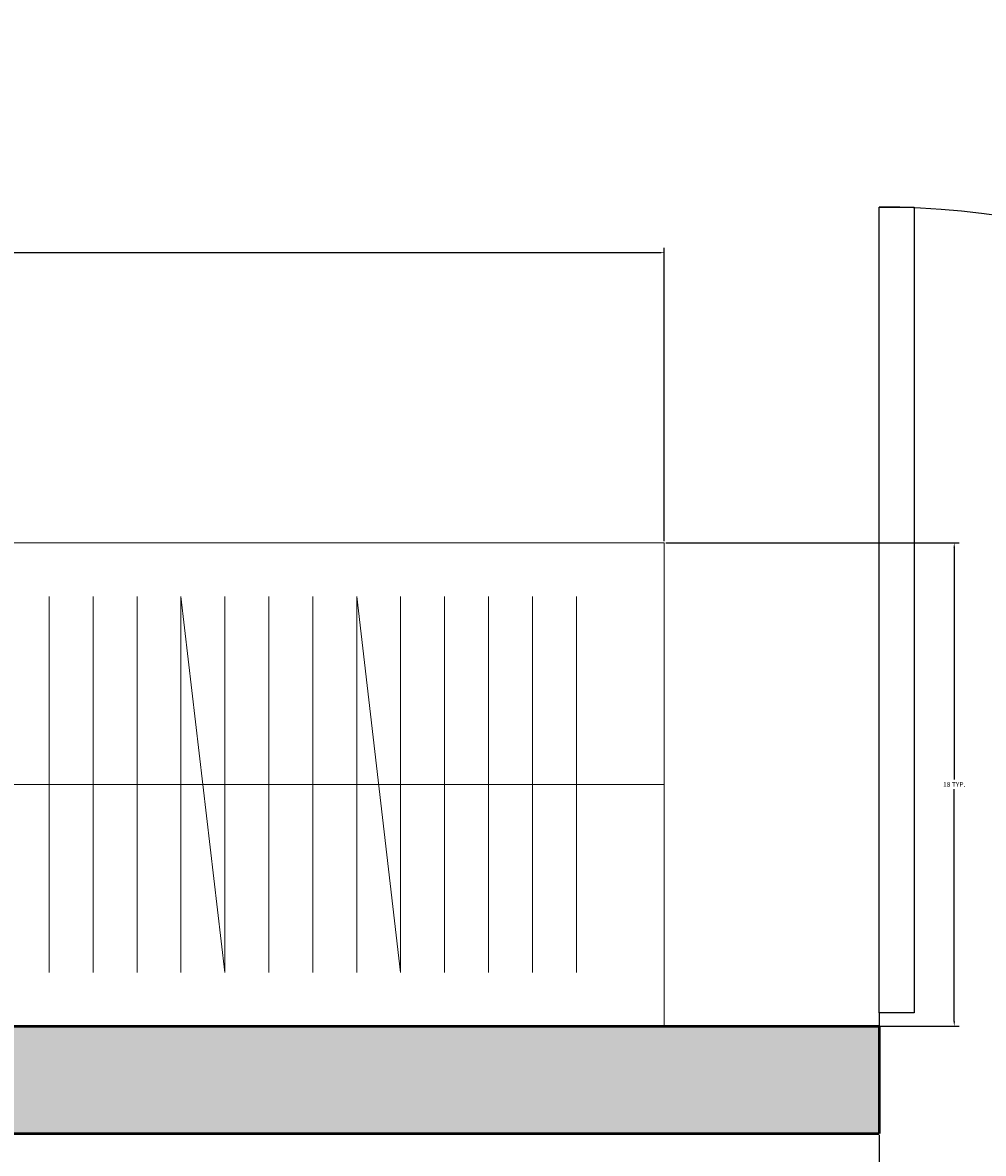
# Model space of a CAD drawing. Units: inches. Extents: x 2307 to 2544, y 2171 to 2540.
# Tile 20 of 52: x 2384 to 2420, y 2387 to 2429. Entities that reach past the tile are written whole.
import ezdxf

# ---------------------------------------------------------------- set-up
doc = ezdxf.new("R2010")
doc.units = ezdxf.units.IN
for name, color, linetype, lineweight in [('A-ANNO-DIMS', 2, 'Continuous', 18), ('A-DOOR', 3, 'Continuous', 25), ('A-FLOR-CASE', 9, 'Continuous', 18), ('A-WALL', 7, 'Continuous', 50)]:
    doc.layers.add(name, color=color, linetype=linetype, lineweight=lineweight)
doc.layers.add('A-WALL-PATT', color=18, linetype='Continuous', lineweight=13, true_color=0x000000)
doc.styles.get("Standard").update_dxf_attribs({"font": 'arial.ttf'})
doc.dimstyles.get("Standard").update_dxf_attribs({"dimtxt": 0.18, "dimasz": 0.18, "dimexe": 0.18, "dimexo": 0.0625, "dimgap": 0.09, "dimtad": 0, "dimtih": 1, "dimtoh": 1, "dimdec": 4, "dimzin": 0, "dimdsep": 46, "dimtxsty": 'Standard', "dimcen": 0.09, "dimadec": 0, "dimazin": 0, "dimtfac": 1, "dimtdec": 4, "dimtofl": 0, "dimtmove": 0, "dimatfit": 3, "dimfxl": 1, "dimtolj": 1, "dimtzin": 0, "dimarcsym": 0})

# ---------------------------------------------------------------- blocks, each defined once
blk = doc.blocks.new('*U13')
for p, q in [((0, 0), (0, -6)), ((40, 0), (40, -6))]:
    blk.add_line(p, q)
blk.add_lwpolyline([(0, 0), (0, 40), (1.75, 40), (1.75, 0)], close=True)
blk.add_arc((0, 0), 40, 0, 90)
blk = doc.blocks.new('WARDROBE-72X18IN')
for p, q in [((0, 72), (0, 0)), ((9, 72), (9, 0)), ((18, 0), (18, 72)), ((16, 22.909), (2, 22.909)), ((16, 21.272), (2, 21.272)), ((16, 19.636), (2, 19.636)), ((16, 18), (2, 18)), ((16, 18), (2, 16.363)), ((16, 16.363), (2, 16.363)), ((16, 14.727), (2, 14.727)), ((16, 13.09), (2, 13.09)), ((16, 11.454), (2, 11.454)), ((16, 11.454), (2, 9.818)), ((16, 9.818), (2, 9.818)), ((16, 8.181), (2, 8.181)), ((16, 6.545), (2, 6.545)), ((16, 4.909), (2, 4.909)), ((16, 3.272), (2, 3.272)), ((0, 0), (18, 0)), ((18, 0), (0, 0))]:
    blk.add_line(p, q)
blk = doc.blocks.new('*D18')
at = {"layer": 'A-ANNO-DIMS', "color": 0, "lineweight": -2, "transparency": 16777216}
for p, q in [((2335.696, 2409.572), (2335.696, 2420.49)), ((2335.876, 2420.31), (2370.389, 2420.31)), ((2407.516, 2420.31), (2373.003, 2420.31)), ((2407.696, 2409.572), (2407.696, 2420.49))]:
    blk.add_line(p, q, dxfattribs=at)
at = {"layer": 'A-ANNO-DIMS', "color": 0, "transparency": 16777216}
for points in [[(2335.876, 2420.34), (2335.876, 2420.28), (2335.696, 2420.31)], [(2407.516, 2420.34), (2407.516, 2420.28), (2407.696, 2420.31)]]:
    blk.add_solid(points, dxfattribs=at)
at = {"layer": 'Defpoints', "color": 0, "transparency": 16777216}
for p in [(2335.696, 2420.31), (2335.696, 2409.51), (2407.696, 2409.51)]:
    blk.add_point(p, dxfattribs=at)
at = {"layer": 'A-ANNO-DIMS', "color": 0, "transparency": 16777216, "insert": (2371.696, 2420.31), "char_height": 0.18, "attachment_point": 5}
blk.add_mtext('\\A1;WARDROBE 72 TYP.', dxfattribs=at)
blk = doc.blocks.new('*D19')
at = {"layer": 'A-ANNO-DIMS', "color": 0, "lineweight": -2, "transparency": 16777216}
for p, q in [((2407.758, 2409.51), (2418.676, 2409.51)), ((2418.496, 2409.33), (2418.496, 2400.691)), ((2418.496, 2391.69), (2418.496, 2400.328)), ((2407.758, 2391.51), (2418.676, 2391.51))]:
    blk.add_line(p, q, dxfattribs=at)
at = {"layer": 'A-ANNO-DIMS', "color": 0, "transparency": 16777216}
for points in [[(2418.466, 2409.33), (2418.526, 2409.33), (2418.496, 2409.51)], [(2418.466, 2391.69), (2418.526, 2391.69), (2418.496, 2391.51)]]:
    blk.add_solid(points, dxfattribs=at)
at = {"layer": 'Defpoints', "color": 0, "transparency": 16777216}
for p in [(2407.696, 2409.51), (2418.496, 2409.51), (2407.696, 2391.51)]:
    blk.add_point(p, dxfattribs=at)
at = {"layer": 'A-ANNO-DIMS', "color": 0, "transparency": 16777216, "insert": (2418.496, 2400.51), "char_height": 0.18, "attachment_point": 5}
blk.add_mtext('\\A1;18 TYP.', dxfattribs=at)
blk = doc.blocks.new('*D51')
at = {"layer": 'A-ANNO-DIMS', "color": 0, "lineweight": -2, "transparency": 16777216}
for p, q in [((2415.696, 2387.447), (2415.696, 2368.18)), ((2445.696, 2387.447), (2445.696, 2368.18)), ((2415.876, 2368.36), (2430.477, 2368.36)), ((2445.516, 2368.36), (2430.914, 2368.36))]:
    blk.add_line(p, q, dxfattribs=at)
at = {"layer": 'A-ANNO-DIMS', "color": 0, "transparency": 16777216}
for points in [[(2415.876, 2368.39), (2415.876, 2368.33), (2415.696, 2368.36)], [(2445.516, 2368.39), (2445.516, 2368.33), (2445.696, 2368.36)]]:
    blk.add_solid(points, dxfattribs=at)
at = {"layer": 'Defpoints', "color": 0, "transparency": 16777216}
for p in [(2415.696, 2387.51), (2445.696, 2387.51), (2415.696, 2368.36)]:
    blk.add_point(p, dxfattribs=at)
at = {"layer": 'A-ANNO-DIMS', "color": 0, "transparency": 16777216, "insert": (2430.696, 2368.36), "char_height": 0.18, "attachment_point": 5}
blk.add_mtext('\\A1;30', dxfattribs=at)

msp = doc.modelspace()

# ---------------------------------------------------------------- hatches: boundary and pattern name
at = {"layer": 'A-WALL-PATT'}
h = msp.add_hatch(color=256, dxfattribs=at)
h.dxf.hatch_style = 1
h.paths.add_polyline_path([(2367.4028, 2520.5096), (2326.6958, 2520.5096), (2326.6958, 2355.3983), (2335.6958, 2355.3983), (2335.6958, 2387.5096), (2415.6958, 2387.5096), (2415.6958, 2391.5096), (2335.6958, 2391.5096), (2335.6958, 2409.5096), (2335.6958, 2511.5096), (2367.4028, 2511.5096)])

# ---------------------------------------------------------------- linework, layer by layer
at = {"layer": 'A-WALL'}
for p, q in [((2335.6958, 2391.5096), (2415.6958, 2391.5096)), ((2415.6958, 2391.5096), (2415.6958, 2387.5096)), ((2335.6958, 2387.5096), (2415.6958, 2387.5096))]:
    msp.add_line(p, q, dxfattribs=at)

# ---------------------------------------------------------------- block references
at = {"layer": 'A-DOOR', "xscale": 0.75, "yscale": 0.75, "zscale": 0.75}
msp.add_blockref('*U13', (2415.6958, 2392.0096), dxfattribs=at)
at = {"layer": 'A-FLOR-CASE', "rotation": 90.00000000000885}
msp.add_blockref('WARDROBE-72X18IN', (2407.6954, 2391.5097), dxfattribs=at)

# ---------------------------------------------------------------- dimensions: what is measured, and where the dimension line sits
at = {"layer": 'A-ANNO-DIMS'}
for base, p1, p2, angle, text, picture, middle in [((2335.6958, 2420.3096), (2407.6958, 2409.5096), (2335.6958, 2409.5096), 180, 'WARDROBE <> TYP.', '*D18', (2371.6958, 2420.3096)), ((2418.4958, 2409.5096), (2407.6958, 2391.5096), (2407.6958, 2409.5096), 90, '<> TYP.', '*D19', (2418.4958, 2400.5096))]:
    dim = msp.add_linear_dim(base=base, p1=p1, p2=p2, angle=angle, text=text, dimstyle='Standard', override={"dimdec": 0, "dimlfac": 1, "dimrnd": 0, "dimzin": 0, "dimdsep": 46, "dimlunit": 2}, dxfattribs=at)
    dim.commit()
    dim.dimension.update_dxf_attribs({"geometry": picture, "text_midpoint": middle})
dim = msp.add_linear_dim(base=(2415.6958, 2368.3596), p1=(2445.6958, 2387.5096), p2=(2415.6958, 2387.5096), angle=180, dimstyle='Standard', override={"dimdec": 0, "dimlfac": 1, "dimrnd": 0, "dimzin": 0, "dimdsep": 46, "dimlunit": 2}, dxfattribs=at)
dim.commit()
dim.dimension.update_dxf_attribs({"geometry": '*D51', "text_midpoint": (2430.6958, 2368.3596)})

doc.saveas('drawing.dxf')
